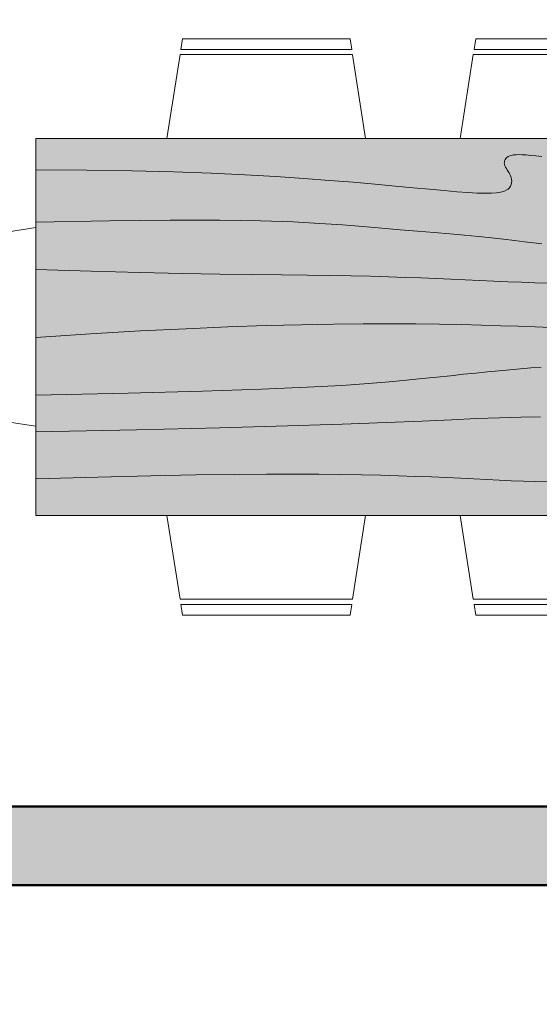
# Model space of a CAD drawing. Units: inches. Extents: x 2419 to 2878, y 1068 to 1713.
# Tile 4 of 20: x 2508 to 2541, y 1286 to 1349. Entities that reach past the tile are written whole.
import ezdxf

# ---------------------------------------------------------------- set-up
doc = ezdxf.new("R2010")
doc.units = ezdxf.units.IN
for name, color, linetype, lineweight in [('A-ANNO-DIMS', 2, 'Continuous', 18), ('A-FLOR-PRKG-PATT', 1, 'Continuous', 13), ('A-FURN', 8, 'Continuous', 18), ('A-FURN-PATT', 254, 'Continuous', 13), ('A-WALL', 7, 'Continuous', 50)]:
    doc.layers.add(name, color=color, linetype=linetype, lineweight=lineweight)
doc.layers.add('A-WALL-PATT', color=18, linetype='Continuous', lineweight=13, true_color=0x000000)
doc.styles.get("Standard").update_dxf_attribs({"font": 'arial.ttf'})
doc.dimstyles.new('ISO-25', dxfattribs={"dimtxt": 12.5, "dimasz": 2.5, "dimexe": 1.25, "dimexo": 0.625, "dimtad": 1, "dimdec": 0, "dimlunit": 4, "dimtxsty": 'Standard', "dimblk": 'ARCHTICK', "dimcen": 2.5, "dimse1": 1, "dimse2": 1, "dimclrd": 4, "dimadec": 0, "dimazin": 0, "dimtfac": 1, "dimtdec": 0, "dimtmove": 0, "dimatfit": 3, "dimfxl": 1, "dimarcsym": 0})

# ---------------------------------------------------------------- blocks, each defined once
blk = doc.blocks.new('Dining Set - 36 x 72 in.')
for p, q in [((-22, 27.5), (-22.1562, 26.50042)), ((-22, 27.5), (-6, 27.5)), ((-5.8437, 26.49966), (-6, 27.5)), ((6, 27.5), (5.8438, 26.50042)), ((6, 27.5), (22, 27.5)), ((-5.8416, 26.5), (-22.1534, 26.5)), ((22.1584, 26.5), (5.8466, 26.5)), ((-22.2343, 26.00059), (-23.4847, 17.99762)), ((-22.2304, 26), (-5.7608, 26)), ((-4.5152, 17.99762), (-5.7655, 25.99926)), ((5.7657, 26.00059), (4.5153, 17.99762)), ((5.7696, 26), (22.2392, 26)), ((36, 18), (-36, 18)), ((-36, 18), (-36, -18)), ((-44.0006, 8.23428), (-35.9976, 9.48474)), ((-35.9976, -9.48476), (-43.9993, -8.2345)), ((-36, -18), (36, -18)), ((-22.2343, -26.0006), (-23.4847, -17.99762)), ((-4.5152, -17.99762), (-5.7655, -25.99928)), ((5.7657, -26.0006), (4.5153, -17.99762)), ((-22.2304, -26), (-5.7608, -26)), ((5.7696, -26), (22.2392, -26)), ((-22, -27.5), (-22.1562, -26.50044)), ((-5.8416, -26.5), (-22.1534, -26.5)), ((-5.8437, -26.49967), (-6, -27.5)), ((6, -27.5), (5.8438, -26.50044)), ((22.1584, -26.5), (5.8466, -26.5)), ((-22, -27.5), (-6, -27.5)), ((6, -27.5), (22, -27.5))]:
    blk.add_line(p, q)
for points in [[(-36, 15), (-31.1772, 14.97754), (-26.8079, 14.91406), (-22.8538, 14.81543), (-19.276, 14.6875), (-16.0362, 14.53613), (-13.0957, 14.36718), (-10.4159, 14.18652), (-7.9583, 14), (-5.6904, 13.81315), (-3.6035, 13.63021), (-1.6954, 13.45508), (0.0365, 13.29166), (1.5945, 13.14388), (2.9811, 13.01562), (4.1988, 12.9108), (5.25, 12.83333), (6.1393, 12.78613), (6.8802, 12.76823), (7.4883, 12.77767), (7.9792, 12.8125), (8.3685, 12.87077), (8.6719, 12.95052), (8.9049, 13.0498), (9.0833, 13.16666), (9.2205, 13.29899), (9.3216, 13.44401), (9.3895, 13.59879), (9.4271, 13.76041), (9.4373, 13.92594), (9.4232, 14.09245), (9.3875, 14.257), (9.3333, 14.41666), (9.2638, 14.56917), (9.1836, 14.71484), (9.0975, 14.85465), (9.0104, 14.98958), (8.9272, 15.1206), (8.8529, 15.2487), (8.7922, 15.37483), (8.75, 15.5), (8.7305, 15.62467), (8.7344, 15.74739), (8.7617, 15.86621), (8.8125, 15.97916), (8.8867, 16.08431), (8.9844, 16.17968), (9.1055, 16.26334), (9.25, 16.33333), (9.4189, 16.38802), (9.6172, 16.42708), (9.8506, 16.45052), (10.125, 16.45833), (10.4463, 16.45052), (10.8203, 16.42708), (11.2529, 16.38802), (11.75, 16.33333), (12.3184, 16.26318)], [(-36, 10), (-28.9766, 10.14274), (-23.1725, 10.20442), (-18.4241, 10.19775), (-14.5677, 10.13541), (-11.4399, 10.03011), (-8.877, 9.89453), (-6.7154, 9.74137), (-4.7917, 9.58333), (-2.9698, 9.43082), (-1.2246, 9.28515), (0.4415, 9.14534), (2.026, 9.01041), (3.5266, 8.87939), (4.9408, 8.7513), (6.266, 8.62516), (7.5, 8.5), (8.6411, 8.37549), (9.6914, 8.2539), (10.6538, 8.13818), (11.5312, 8.03125), (12.3267, 7.93603)], [(-36, 5.5), (-30.7157, 5.3348), (-26.069, 5.20963), (-21.9946, 5.11767), (-18.4271, 5.05208), (-15.3009, 5.00602), (-12.5508, 4.97265), (-10.1112, 4.94515), (-7.9167, 4.91666), (-5.909, 4.88167), (-4.0586, 4.83984), (-2.3429, 4.79215), (-0.7396, 4.73958), (0.7739, 4.6831), (2.22, 4.6237), (3.6213, 4.56233), (5, 4.5), (6.373, 4.43782), (7.7344, 4.3776), (9.0723, 4.32129), (10.375, 4.27083), (11.6309, 4.22819), (12.8281, 4.19531)], [(-36, -1), (-30.7915, -0.6591), (-26.0195, -0.38216), (-21.6519, -0.16284), (-17.6563, 0.00521), (-14.0005, 0.12833), (-10.6523, 0.21289), (-7.5796, 0.26522), (-4.75, 0.29166), (-2.134, 0.29793), (0.2878, 0.28711), (2.5317, 0.26163), (4.6146, 0.22396), (6.5529, 0.17651), (8.3633, 0.12174), (10.0623, 0.06209), (11.6667, 0), (13.1899, -0.06201)], [(-36, -6.5), (-27.1843, -6.31267), (-20.084, -6.1263), (-14.469, -5.9419), (-10.1094, -5.76042), (-6.7752, -5.58285), (-4.2363, -5.41016), (-2.2629, -5.24333), (-0.625, -5.08334), (0.8708, -4.93099), (2.2715, -4.78646), (3.5872, -4.64974), (4.8281, -4.52084), (6.0046, -4.39974), (7.127, -4.28646), (8.2053, -4.18099), (9.25, -4.08334), (10.2705, -3.99382), (11.2734, -3.91407), (12.2647, -3.84603)], [(-36, -10), (-26.4022, -9.81299), (-18.4675, -9.62891), (-11.9839, -9.45069), (-6.7396, -9.28125), (-2.5226, -9.12354), (0.8789, -8.98047), (3.6769, -8.85498), (6.0833, -8.75), (8.2767, -8.66765), (10.3021, -8.60677), (12.1712, -8.56543)], [(-36, -14.5), (-30.0881, -14.33513), (-25.0332, -14.21224), (-20.7312, -14.12647), (-17.0781, -14.07292), (-13.97, -14.04671), (-11.3027, -14.04297), (-8.9724, -14.05681), (-6.875, -14.08334), (-4.9224, -14.11833), (-3.0905, -14.16016), (-1.3709, -14.20785), (0.2448, -14.26042), (1.7647, -14.3169), (3.1973, -14.3763), (4.5507, -14.43767), (5.8333, -14.5), (7.0554, -14.5621), (8.235, -14.62175), (9.3922, -14.67652), (10.5469, -14.72396), (11.7192, -14.76164), (12.929, -14.78711)]]:
    blk.add_lwpolyline(points)
blk = doc.blocks.new('_ArchTick')
at = {"color": 0, "linetype": 'ByBlock', "const_width": 0.15}
blk.add_lwpolyline([(-0.5, -0.5), (0.5, 0.5)], dxfattribs=at)
blk = doc.blocks.new('*D26')
at = {"layer": 'A-ANNO-DIMS', "color": 4, "lineweight": -2, "transparency": 16777216}
for p, q in [((2502.769, 1356.79), (2563.458, 1356.79)), ((2563.458, 1356.79), (2733.724, 1356.79))]:
    blk.add_line(p, q, dxfattribs=at)
at = {"layer": 'Defpoints', "color": 0, "transparency": 16777216}
for p in [(2563.458, 1356.79), (2502.769, 1347.687), (2563.458, 1347.687)]:
    blk.add_point(p, dxfattribs=at)
at = {"layer": 'A-ANNO-DIMS', "color": 4, "lineweight": -2, "transparency": 16777216, "xscale": 2.5, "yscale": 2.5, "zscale": 2.5, "rotation": 180}
blk.add_blockref('_ArchTick', (2502.769, 1356.79), dxfattribs=at)
at = {"layer": 'A-ANNO-DIMS', "color": 4, "lineweight": -2, "transparency": 16777216, "xscale": 2.5, "yscale": 2.5, "zscale": 2.5}
blk.add_blockref('_ArchTick', (2563.458, 1356.79), dxfattribs=at)
at = {"layer": 'A-ANNO-DIMS', "color": 0, "transparency": 16777216, "insert": (2649.841, 1363.878), "char_height": 12.5, "attachment_point": 5}
blk.add_mtext('DINING SET 5\'-0 1/2"', dxfattribs=at)
blk = doc.blocks.new('*D43')
at = {"layer": 'A-ANNO-DIMS', "color": 4, "lineweight": -2, "transparency": 16777216}
blk.add_line((2480.514, 1079.925), (2557.299, 1079.925), dxfattribs=at)
at = {"layer": 'Defpoints', "color": 0, "transparency": 16777216}
for p in [(2480.514, 1408.813), (2557.299, 1408.813), (2557.299, 1079.925)]:
    blk.add_point(p, dxfattribs=at)
at = {"layer": 'A-ANNO-DIMS', "color": 4, "lineweight": -2, "transparency": 16777216, "xscale": 2.5, "yscale": 2.5, "zscale": 2.5, "rotation": 180}
blk.add_blockref('_ArchTick', (2480.514, 1079.925), dxfattribs=at)
at = {"layer": 'A-ANNO-DIMS', "color": 4, "lineweight": -2, "transparency": 16777216, "xscale": 2.5, "yscale": 2.5, "zscale": 2.5}
blk.add_blockref('_ArchTick', (2557.299, 1079.925), dxfattribs=at)
at = {"layer": 'A-ANNO-DIMS', "color": 0, "transparency": 16777216, "insert": (2518.907, 1086.932), "char_height": 12.5, "attachment_point": 5}
blk.add_mtext('6\'-5"', dxfattribs=at)
blk = doc.blocks.new('*D47')
at = {"layer": 'A-ANNO-DIMS', "color": 4, "lineweight": -2, "transparency": 16777216}
for p, q in [((2444.314, 1376.561), (2444.314, 1357.976)), ((2444.314, 1357.976), (2444.314, 1293.048))]:
    blk.add_line(p, q, dxfattribs=at)
at = {"layer": 'Defpoints', "color": 0, "transparency": 16777216}
for p in [(2632.514, 1376.561), (2444.314, 1357.976), (2632.514, 1357.976)]:
    blk.add_point(p, dxfattribs=at)
at = {"layer": 'A-ANNO-DIMS', "color": 4, "lineweight": -2, "transparency": 16777216, "xscale": 2.5, "yscale": 2.5, "zscale": 2.5}
for p, rotation in [((2444.314, 1376.561), 90), ((2444.314, 1357.976), 270)]:
    blk.add_blockref('_ArchTick', p, dxfattribs=dict(at, rotation=rotation))
at = {"layer": 'A-ANNO-DIMS', "color": 0, "transparency": 16777216, "insert": (2437.226, 1324.262), "char_height": 12.5, "attachment_point": 5, "rotation": 90}
blk.add_mtext('1\'-6 1/2"', dxfattribs=at)
blk = doc.blocks.new('*D56')
at = {"layer": 'A-ANNO-DIMS', "color": 4, "lineweight": -2, "transparency": 16777216}
for p, q in [((2480.514, 1079.925), (2503.967, 1079.925)), ((2503.967, 1079.925), (2578.607, 1079.925))]:
    blk.add_line(p, q, dxfattribs=at)
at = {"layer": 'Defpoints', "color": 0, "transparency": 16777216}
for p in [(2480.514, 1507.813), (2503.967, 1494.852), (2503.967, 1079.925)]:
    blk.add_point(p, dxfattribs=at)
at = {"layer": 'A-ANNO-DIMS', "color": 4, "lineweight": -2, "transparency": 16777216, "xscale": 2.5, "yscale": 2.5, "zscale": 2.5, "rotation": 180}
blk.add_blockref('_ArchTick', (2480.514, 1079.925), dxfattribs=at)
at = {"layer": 'A-ANNO-DIMS', "color": 4, "lineweight": -2, "transparency": 16777216, "xscale": 2.5, "yscale": 2.5, "zscale": 2.5}
blk.add_blockref('_ArchTick', (2503.967, 1079.925), dxfattribs=at)
at = {"layer": 'A-ANNO-DIMS', "color": 0, "transparency": 16777216, "insert": (2542.537, 1087.013), "char_height": 12.5, "attachment_point": 5}
blk.add_mtext('1\'-11 1/2"', dxfattribs=at)
blk = doc.blocks.new('*D59')
at = {"layer": 'A-ANNO-DIMS', "color": 4, "lineweight": -2, "transparency": 16777216}
blk.add_line((2480.514, 1079.925), (2589.514, 1079.925), dxfattribs=at)
at = {"layer": 'Defpoints', "color": 0, "transparency": 16777216}
for p in [(2480.514, 1414.813), (2589.514, 1414.813), (2589.514, 1079.925)]:
    blk.add_point(p, dxfattribs=at)
at = {"layer": 'A-ANNO-DIMS', "color": 4, "lineweight": -2, "transparency": 16777216, "xscale": 2.5, "yscale": 2.5, "zscale": 2.5, "rotation": 180}
blk.add_blockref('_ArchTick', (2480.514, 1079.925), dxfattribs=at)
at = {"layer": 'A-ANNO-DIMS', "color": 4, "lineweight": -2, "transparency": 16777216, "xscale": 2.5, "yscale": 2.5, "zscale": 2.5}
blk.add_blockref('_ArchTick', (2589.514, 1079.925), dxfattribs=at)
at = {"layer": 'A-ANNO-DIMS', "color": 0, "transparency": 16777216, "insert": (2535.014, 1086.932), "char_height": 12.5, "attachment_point": 5}
blk.add_mtext('9\'-1"', dxfattribs=at)

msp = doc.modelspace()

# ---------------------------------------------------------------- hatches: boundary and pattern name
at = {"layer": 'A-FLOR-PRKG-PATT'}
h = msp.add_hatch(color=256, dxfattribs=at)
h.dxf.hatch_style = 1
edge = h.paths.add_edge_path()
edge.add_ellipse((2561.374, 1279.453), major_axis=(3.988, 0), ratio=0.842304, start_angle=0.64655, end_angle=90)
edge.add_line((2561.374, 1282.813), (2511.571, 1282.813))
edge.add_ellipse((2511.571, 1279.453), major_axis=(3.988, 0), ratio=0.842304, start_angle=90, end_angle=179.35345)
edge.add_ellipse((10560.892, 1188.617), major_axis=(-8054.031, 0), ratio=0.84230387, start_angle=-0.6465541, end_angle=-0.6282372)
edge.add_ellipse((2509.23, 1276.906), major_axis=(1.687, 0), ratio=0.842304, start_angle=179.37176, end_angle=248.46476)
edge.add_ellipse((10560.329, 1188.617), major_axis=(8052.293, 0), ratio=0.84230387, start_angle=179.3534459, end_angle=179.3813568, ccw=False)
edge.add_ellipse((2511.008, 1279.453), major_axis=(2.25, 0), ratio=0.842304, start_angle=90, end_angle=179.35345, ccw=False)
edge.add_line((2511.008, 1281.348), (2561.936, 1281.348))
edge.add_ellipse((2561.936, 1279.453), major_axis=(-2.25, 0), ratio=0.842304, start_angle=180.64655, end_angle=270, ccw=False)
edge.add_ellipse((-5487.385, 1188.617), major_axis=(8052.293, 0), ratio=0.84230387, start_angle=0.5282715, end_angle=0.6465541, ccw=False)
edge.add_ellipse((2563.715, 1276.906), major_axis=(-1.687, 0), ratio=0.842304, start_angle=111.53524, end_angle=180.62824)
edge.add_ellipse((-5487.947, 1188.617), major_axis=(-8054.031, 0), ratio=0.84230387, start_angle=180.6282372, end_angle=180.6465541)
edge = h.paths.add_edge_path()
edge.add_ellipse((2564.908, 1261.91), major_axis=(-1.125, 0), ratio=0.842304, start_angle=180, end_angle=270)
edge.add_line((2564.908, 1262.857), (2564.426, 1262.857))
edge.add_ellipse((-5487.385, 1188.617), major_axis=(8052.293, 0), ratio=0.84230387, start_angle=0.3838668, end_angle=0.5282715, ccw=False)
edge.add_line((2564.654, 1242.564), (2564.908, 1242.564))
edge.add_ellipse((2564.908, 1243.512), major_axis=(-1.125, 0), ratio=0.842304, start_angle=90, end_angle=180)
edge.add_line((2566.033, 1243.512), (2566.033, 1261.91))
edge = h.paths.add_edge_path()
edge.add_ellipse((2564.908, 1174.989), major_axis=(1.125, 0), ratio=0.842304, start_angle=0, end_angle=90)
edge.add_line((2564.908, 1175.936), (2564.894, 1175.936))
edge.add_ellipse((-5487.385, 1188.617), major_axis=(8052.293, 0), ratio=0.84230387, start_angle=-0.1349866, end_angle=-0.0902291, ccw=False)
edge.add_ellipse((2163.343, 1170.913), major_axis=(401.537, 0), ratio=0.8423039, start_angle=-2.17995, end_angle=-0.13561, ccw=False)
edge.add_line((2564.47, 1155.643), (2564.908, 1155.643))
edge.add_ellipse((2564.908, 1156.591), major_axis=(-1.125, 0), ratio=0.842304, start_angle=90, end_angle=180)
edge.add_line((2566.033, 1156.591), (2566.033, 1174.989))
h.paths.add_polyline_path([(2574.476, 1207.448), (2633.94, 1207.448), (2633.94, 1217.366), (2574.476, 1217.366)], flags=9)
h.paths.add_polyline_path([(2574.454, 1217.828), (2610.472, 1217.828), (2610.472, 1227.879), (2574.454, 1227.879)], flags=9)
h.paths.add_polyline_path([(2672.426, 1304.02), (2718.617, 1304.02), (2718.617, 1313.939), (2672.426, 1313.939)], flags=9)
h.paths.add_polyline_path([(2672.404, 1314.4), (2750.128, 1314.4), (2750.128, 1324.451), (2672.404, 1324.451)], flags=9)
h.paths.add_polyline_path([(2500.432, 1374.444), (2544.803, 1374.444), (2544.803, 1384.362), (2500.432, 1384.362)], flags=9)
h.paths.add_polyline_path([(2500.41, 1384.824), (2566.075, 1384.824), (2566.075, 1394.875), (2500.41, 1394.875)], flags=9)
h.paths.add_polyline_path([(2738.933, 1376.749), (2778.273, 1376.749), (2778.273, 1386.667), (2738.933, 1386.667)], flags=9)
h.paths.add_polyline_path([(2659.12, 1357.8), (2703.492, 1357.8), (2703.492, 1367.718), (2659.12, 1367.718)], flags=9)
h.paths.add_polyline_path([(2659.098, 1368.18), (2694.114, 1368.18), (2694.114, 1378.23), (2659.098, 1378.23)], flags=9)
h.paths.add_polyline_path([(2730.123, 1466.067), (2769.463, 1466.067), (2769.463, 1475.986), (2730.123, 1475.986)], flags=9)
h.paths.add_polyline_path([(2730.101, 1476.447), (2765.117, 1476.447), (2765.117, 1486.498), (2730.101, 1486.498)], flags=9)
h.paths.add_polyline_path([(2730.382, 1518.647), (2761.48, 1518.647), (2761.48, 1528.566), (2730.382, 1528.566)], flags=9)
h.paths.add_polyline_path([(2730.361, 1529.028), (2780.958, 1529.028), (2780.958, 1539.072), (2730.361, 1539.072)], flags=9)
h.paths.add_polyline_path([(2629.32, 1455.189), (2688.784, 1455.189), (2688.784, 1465.107), (2629.32, 1465.107)], flags=9)
h.paths.add_polyline_path([(2629.298, 1465.569), (2681.902, 1465.569), (2681.902, 1475.62), (2629.298, 1475.62)], flags=9)
h.paths.add_polyline_path([(2513.229, 1456.484), (2562.631, 1456.484), (2562.631, 1466.402), (2513.229, 1466.402)], flags=9)
h.paths.add_polyline_path([(2513.208, 1466.865), (2556.26, 1466.865), (2556.26, 1476.909), (2513.208, 1476.909)], flags=9)
h.paths.add_polyline_path([(2488.87, 1521.538), (2519.968, 1521.538), (2519.968, 1531.456), (2488.87, 1531.456)], flags=9)
h.paths.add_polyline_path([(2536.549, 1543.507), (2580.923, 1543.507), (2580.923, 1553.432), (2536.549, 1553.432)], flags=9)
h.paths.add_polyline_path([(2536.557, 1553.921), (2573.525, 1553.921), (2573.525, 1563.8), (2536.557, 1563.8)], flags=9)
at = {"layer": 'A-FURN-PATT'}
h = msp.add_hatch(color=256, dxfattribs=at)
h.dxf.hatch_style = 1
h.paths.add_polyline_path([(2541.329, 1340.193), (2541.763, 1340.136), (2542.26, 1340.071), (2542.829, 1339.996), (2543.477, 1339.914), (2544.213, 1339.825), (2545.044, 1339.73), (2545.979, 1339.628), (2547.025, 1339.521), (2548.178, 1339.41), (2549.434, 1339.295), (2550.79, 1339.177), (2552.241, 1339.056), (2553.783, 1338.933), (2555.412, 1338.808), (2557.123, 1338.683), (2557.123, 1341.351), (2509.104, 1341.351), (2509.104, 1339.35), (2512.321, 1339.335), (2515.235, 1339.293), (2517.872, 1339.227), (2520.258, 1339.142), (2522.419, 1339.041), (2524.38, 1338.928), (2526.167, 1338.808), (2527.806, 1338.683), (2529.318, 1338.559), (2530.71, 1338.437), (2531.983, 1338.32), (2533.138, 1338.211), (2534.177, 1338.112), (2535.102, 1338.027), (2535.914, 1337.957), (2536.615, 1337.905), (2537.208, 1337.874), (2537.702, 1337.862), (2538.108, 1337.868), (2538.435, 1337.891), (2538.695, 1337.93), (2538.897, 1337.983), (2539.052, 1338.05), (2539.171, 1338.128), (2539.263, 1338.216), (2539.33, 1338.313), (2539.376, 1338.416), (2539.401, 1338.524), (2539.407, 1338.634), (2539.398, 1338.745), (2539.374, 1338.855), (2539.338, 1338.961), (2539.292, 1339.063), (2539.238, 1339.16), (2539.211, 1339.204), (2538.872, 1339.739), (2539.045, 1340.125), (2539.381, 1340.287), (2539.76, 1340.325), (2540.185, 1340.315), (2540.752, 1340.264)])
h.paths.add_polyline_path([(2557.123, 1329.334), (2556.881, 1329.353), (2556.861, 1329.358), (2556.848, 1329.36), (2556.516, 1329.438), (2556.428, 1329.458), (2556.199, 1329.504), (2555.916, 1329.558), (2555.589, 1329.615), (2555.23, 1329.673), (2554.848, 1329.728), (2554.455, 1329.778), (2554.061, 1329.819), (2553.677, 1329.847), (2553.311, 1329.86), (2552.963, 1329.859), (2552.628, 1329.845), (2552.301, 1329.819), (2551.98, 1329.783), (2551.66, 1329.737), (2551.338, 1329.684), (2551.009, 1329.624), (2550.353, 1329.499), (2549.707, 1329.384), (2549.089, 1329.301), (2548.61, 1329.249), (2548.085, 1329.208), (2547.508, 1329.18), (2546.875, 1329.166), (2546.185, 1329.167), (2545.44, 1329.179), (2544.639, 1329.201), (2543.783, 1329.23), (2542.873, 1329.266), (2541.91, 1329.305), (2540.894, 1329.346), (2539.824, 1329.388), (2538.691, 1329.428), (2537.484, 1329.464), (2536.191, 1329.496), (2534.802, 1329.521), (2533.305, 1329.538), (2531.69, 1329.545), (2529.946, 1329.541), (2528.058, 1329.523), (2526.009, 1329.488), (2523.776, 1329.432), (2521.338, 1329.35), (2518.673, 1329.238), (2515.761, 1329.092), (2512.578, 1328.907), (2509.104, 1328.68), (2509.104, 1325.012), (2514.984, 1325.136), (2519.719, 1325.261), (2523.464, 1325.384), (2526.371, 1325.505), (2528.595, 1325.623), (2530.288, 1325.738), (2531.604, 1325.85), (2532.697, 1325.956), (2533.694, 1326.058), (2534.628, 1326.154), (2535.506, 1326.245), (2536.333, 1326.331), (2537.118, 1326.412), (2537.867, 1326.488), (2538.586, 1326.558), (2539.282, 1326.623), (2539.963, 1326.683), (2540.632, 1326.736), (2541.293, 1326.782), (2541.95, 1326.818), (2542.607, 1326.844), (2543.268, 1326.858), (2543.937, 1326.859), (2544.618, 1326.846), (2545.312, 1326.817), (2546.015, 1326.775), (2546.719, 1326.721), (2547.418, 1326.658), (2548.103, 1326.587), (2548.768, 1326.509), (2549.406, 1326.428), (2550.009, 1326.345), (2550.572, 1326.262), (2551.1, 1326.179), (2551.597, 1326.097), (2552.069, 1326.015), (2552.521, 1325.935), (2552.959, 1325.857), (2553.389, 1325.78), (2553.816, 1325.706), (2554.244, 1325.636), (2554.672, 1325.573), (2555.099, 1325.524), (2555.521, 1325.494), (2555.937, 1325.489), (2556.344, 1325.515), (2556.74, 1325.576), (2557.123, 1325.678)])
h.paths.add_polyline_path([(2557.123, 1335.349), (2555.251, 1335.701), (2553.623, 1336.012), (2552.215, 1336.285), (2551.006, 1336.526), (2549.972, 1336.74), (2549.092, 1336.931), (2548.343, 1337.105), (2547.702, 1337.266), (2547.15, 1337.418), (2546.674, 1337.56), (2546.265, 1337.69), (2545.913, 1337.805), (2545.61, 1337.903), (2545.346, 1337.981), (2545.111, 1338.039), (2544.896, 1338.072), (2544.693, 1338.08), (2544.502, 1338.065), (2544.326, 1338.029), (2544.166, 1337.975), (2544.025, 1337.905), (2543.903, 1337.822), (2543.804, 1337.729), (2543.729, 1337.627), (2543.679, 1337.521), (2543.653, 1337.409), (2543.649, 1337.294), (2543.666, 1337.176), (2543.701, 1337.055), (2543.752, 1336.932), (2543.818, 1336.808), (2543.895, 1336.683), (2543.983, 1336.558), (2544.078, 1336.433), (2544.175, 1336.307), (2544.271, 1336.182), (2544.361, 1336.057), (2544.442, 1335.932), (2544.511, 1335.807), (2544.562, 1335.682), (2544.594, 1335.557), (2544.605, 1335.434), (2544.597, 1335.313), (2544.569, 1335.196), (2544.524, 1335.084), (2544.461, 1334.979), (2544.381, 1334.881), (2544.284, 1334.793), (2544.172, 1334.715), (2544.039, 1334.648), (2543.884, 1334.593), (2543.701, 1334.55), (2543.487, 1334.52), (2543.237, 1334.504), (2542.949, 1334.502), (2542.617, 1334.515), (2542.239, 1334.543), (2541.812, 1334.585), (2541.334, 1334.639), (2540.804, 1334.703), (2540.219, 1334.774), (2539.577, 1334.851), (2538.876, 1334.932), (2538.115, 1335.015), (2537.292, 1335.099), (2536.409, 1335.183), (2535.465, 1335.268), (2534.465, 1335.356), (2533.408, 1335.446), (2532.297, 1335.539), (2531.133, 1335.636), (2529.918, 1335.738), (2528.635, 1335.843), (2527.193, 1335.945), (2525.484, 1336.036), (2523.398, 1336.106), (2520.826, 1336.148), (2517.659, 1336.152), (2513.788, 1336.111), (2509.104, 1336.016), (2509.104, 1333.015), (2512.629, 1332.904), (2515.728, 1332.821), (2518.445, 1332.76), (2520.824, 1332.716), (2522.909, 1332.685), (2524.743, 1332.663), (2526.37, 1332.645), (2527.834, 1332.626), (2529.173, 1332.602), (2530.407, 1332.574), (2531.551, 1332.542), (2532.62, 1332.507), (2533.63, 1332.47), (2534.594, 1332.43), (2535.529, 1332.389), (2536.448, 1332.348), (2537.364, 1332.306), (2538.272, 1332.266), (2539.164, 1332.228), (2540.033, 1332.195), (2540.87, 1332.166), (2541.669, 1332.144), (2542.42, 1332.13), (2543.117, 1332.125), (2543.754, 1332.131), (2544.33, 1332.146), (2544.851, 1332.172), (2545.32, 1332.209), (2545.738, 1332.256), (2546.111, 1332.313), (2546.44, 1332.381), (2546.73, 1332.459), (2546.983, 1332.547), (2547.206, 1332.644), (2547.402, 1332.747), (2547.577, 1332.855), (2547.737, 1332.965), (2547.886, 1333.076), (2548.031, 1333.186), (2548.175, 1333.292), (2548.324, 1333.394), (2548.48, 1333.489), (2548.645, 1333.576), (2548.821, 1333.654), (2549.01, 1333.721), (2549.214, 1333.777), (2549.435, 1333.82), (2549.675, 1333.848), (2549.936, 1333.861), (2550.215, 1333.859), (2550.511, 1333.843), (2550.822, 1333.813), (2551.146, 1333.771), (2551.481, 1333.715), (2551.825, 1333.648), (2552.176, 1333.57), (2552.537, 1333.481), (2552.926, 1333.379), (2553.365, 1333.262), (2553.878, 1333.126), (2554.488, 1332.969), (2555.217, 1332.789), (2556.087, 1332.583), (2557.123, 1332.348)])
h.paths.add_polyline_path([(2543.679, 1337.521), (2543.729, 1337.627), (2543.804, 1337.729), (2543.903, 1337.822), (2544.025, 1337.905), (2544.166, 1337.975), (2544.326, 1338.029), (2544.502, 1338.065), (2544.693, 1338.08), (2544.896, 1338.072), (2545.111, 1338.039), (2545.346, 1337.981), (2545.61, 1337.903), (2545.913, 1337.805), (2546.265, 1337.69), (2546.674, 1337.56), (2547.15, 1337.418), (2547.702, 1337.266), (2548.343, 1337.105), (2549.092, 1336.931), (2549.972, 1336.74), (2551.006, 1336.526), (2552.215, 1336.285), (2553.623, 1336.012), (2555.251, 1335.701), (2557.123, 1335.349), (2557.123, 1338.683), (2555.412, 1338.808), (2553.783, 1338.933), (2552.241, 1339.056), (2550.79, 1339.177), (2549.434, 1339.295), (2548.178, 1339.41), (2547.025, 1339.521), (2545.979, 1339.628), (2545.044, 1339.73), (2544.213, 1339.825), (2543.477, 1339.914), (2542.829, 1339.996), (2542.26, 1340.071), (2541.763, 1340.136), (2541.329, 1340.193), (2540.95, 1340.24), (2540.618, 1340.276), (2540.33, 1340.302), (2540.08, 1340.318), (2539.866, 1340.323), (2539.683, 1340.318), (2539.527, 1340.302), (2539.395, 1340.276), (2539.282, 1340.24), (2539.186, 1340.193), (2539.105, 1340.137), (2539.04, 1340.073), (2538.991, 1340.003), (2538.957, 1339.928), (2538.939, 1339.849), (2538.936, 1339.767), (2538.949, 1339.684), (2538.977, 1339.6), (2539.018, 1339.516), (2539.067, 1339.431), (2539.123, 1339.343), (2539.222, 1339.189), (2539.323, 1339.007), (2539.374, 1338.855), (2539.398, 1338.745), (2539.407, 1338.634), (2539.401, 1338.524), (2539.376, 1338.416), (2539.33, 1338.313), (2539.263, 1338.216), (2539.171, 1338.128), (2539.052, 1338.05), (2538.897, 1337.983), (2538.695, 1337.93), (2538.435, 1337.891), (2538.108, 1337.868), (2537.702, 1337.862), (2537.208, 1337.874), (2536.615, 1337.905), (2535.914, 1337.957), (2535.102, 1338.027), (2534.177, 1338.112), (2533.138, 1338.211), (2531.983, 1338.32), (2530.71, 1338.437), (2529.318, 1338.559), (2527.806, 1338.683), (2526.167, 1338.808), (2524.38, 1338.928), (2522.419, 1339.041), (2520.258, 1339.142), (2517.872, 1339.227), (2515.235, 1339.293), (2512.321, 1339.335), (2509.104, 1339.35), (2509.104, 1336.016), (2513.788, 1336.111), (2517.659, 1336.152), (2520.826, 1336.148), (2523.398, 1336.106), (2525.484, 1336.036), (2527.193, 1335.945), (2528.635, 1335.843), (2529.918, 1335.738), (2531.133, 1335.636), (2532.297, 1335.539), (2533.408, 1335.446), (2534.465, 1335.356), (2535.465, 1335.268), (2536.409, 1335.183), (2537.292, 1335.099), (2538.115, 1335.015), (2538.876, 1334.932), (2539.577, 1334.851), (2540.219, 1334.774), (2540.804, 1334.703), (2541.334, 1334.639), (2541.812, 1334.585), (2542.239, 1334.543), (2542.617, 1334.515), (2542.949, 1334.502), (2543.237, 1334.504), (2543.487, 1334.52), (2543.701, 1334.55), (2543.884, 1334.593), (2544.039, 1334.648), (2544.172, 1334.715), (2544.284, 1334.793), (2544.381, 1334.881), (2544.461, 1334.979), (2544.524, 1335.084), (2544.569, 1335.196), (2544.597, 1335.313), (2544.605, 1335.434), (2544.594, 1335.557), (2544.562, 1335.682), (2544.511, 1335.807), (2544.442, 1335.932), (2544.361, 1336.057), (2544.271, 1336.182), (2544.175, 1336.307), (2544.078, 1336.433), (2543.983, 1336.558), (2543.895, 1336.683), (2543.818, 1336.808), (2543.752, 1336.932), (2543.701, 1337.055), (2543.666, 1337.176), (2543.649, 1337.294), (2543.653, 1337.409)])
h.paths.add_polyline_path([(2557.123, 1332.348), (2556.087, 1332.583), (2555.217, 1332.789), (2554.488, 1332.969), (2553.878, 1333.126), (2553.365, 1333.262), (2552.926, 1333.379), (2552.537, 1333.481), (2552.176, 1333.57), (2551.825, 1333.648), (2551.481, 1333.715), (2551.146, 1333.771), (2550.822, 1333.813), (2550.511, 1333.843), (2550.215, 1333.859), (2549.936, 1333.861), (2549.675, 1333.848), (2549.435, 1333.82), (2549.214, 1333.777), (2549.01, 1333.721), (2548.821, 1333.654), (2548.645, 1333.576), (2548.48, 1333.489), (2548.324, 1333.394), (2548.175, 1333.292), (2548.031, 1333.186), (2547.886, 1333.076), (2547.737, 1332.965), (2547.577, 1332.855), (2547.402, 1332.747), (2547.206, 1332.644), (2546.983, 1332.547), (2546.73, 1332.459), (2546.44, 1332.381), (2546.111, 1332.313), (2545.738, 1332.256), (2545.32, 1332.209), (2544.851, 1332.172), (2544.33, 1332.146), (2543.754, 1332.131), (2543.117, 1332.125), (2542.42, 1332.13), (2541.669, 1332.144), (2540.87, 1332.166), (2540.033, 1332.195), (2539.164, 1332.228), (2538.272, 1332.266), (2537.364, 1332.306), (2536.448, 1332.348), (2535.529, 1332.389), (2534.594, 1332.43), (2533.63, 1332.47), (2532.62, 1332.507), (2531.551, 1332.542), (2530.407, 1332.574), (2529.173, 1332.602), (2527.834, 1332.626), (2526.37, 1332.645), (2524.743, 1332.663), (2522.909, 1332.685), (2520.824, 1332.716), (2518.445, 1332.76), (2515.728, 1332.821), (2512.629, 1332.904), (2509.104, 1333.015), (2509.104, 1328.68), (2512.578, 1328.907), (2515.761, 1329.092), (2518.673, 1329.238), (2521.338, 1329.35), (2523.776, 1329.432), (2526.009, 1329.488), (2528.058, 1329.523), (2529.946, 1329.541), (2531.69, 1329.545), (2533.305, 1329.538), (2534.802, 1329.521), (2536.191, 1329.496), (2537.484, 1329.464), (2538.691, 1329.428), (2539.824, 1329.388), (2540.894, 1329.346), (2541.91, 1329.305), (2542.873, 1329.266), (2543.783, 1329.23), (2544.639, 1329.201), (2545.44, 1329.179), (2546.185, 1329.167), (2546.875, 1329.166), (2547.508, 1329.18), (2548.085, 1329.208), (2548.61, 1329.249), (2549.089, 1329.301), (2549.529, 1329.36), (2549.936, 1329.425), (2550.314, 1329.492), (2550.67, 1329.56), (2551.009, 1329.624), (2551.338, 1329.684), (2551.66, 1329.737), (2551.98, 1329.783), (2552.301, 1329.819), (2552.628, 1329.845), (2552.963, 1329.859), (2553.311, 1329.86), (2553.677, 1329.847), (2554.061, 1329.819), (2554.455, 1329.778), (2554.848, 1329.728), (2555.23, 1329.673), (2555.589, 1329.615), (2555.916, 1329.558), (2556.199, 1329.504), (2556.428, 1329.458), (2556.596, 1329.421), (2556.712, 1329.393), (2556.792, 1329.374), (2556.848, 1329.36), (2556.895, 1329.352), (2556.948, 1329.348), (2557.019, 1329.347), (2557.123, 1329.346)])
h.paths.add_polyline_path([(2557.123, 1323.011), (2556.483, 1323.018), (2555.818, 1323.039), (2555.136, 1323.071), (2554.441, 1323.111), (2553.741, 1323.159), (2553.043, 1323.21), (2552.352, 1323.263), (2551.676, 1323.316), (2551.018, 1323.367), (2550.371, 1323.415), (2549.725, 1323.46), (2549.071, 1323.501), (2548.398, 1323.538), (2547.698, 1323.57), (2546.96, 1323.599), (2546.174, 1323.622), (2545.331, 1323.64), (2544.423, 1323.652), (2543.442, 1323.655), (2542.381, 1323.65), (2541.231, 1323.634), (2539.984, 1323.606), (2538.633, 1323.566), (2537.171, 1323.511), (2535.566, 1323.441), (2533.7, 1323.357), (2531.431, 1323.262), (2528.619, 1323.157), (2525.121, 1323.044), (2520.797, 1322.925), (2515.505, 1322.802), (2509.104, 1322.677), (2509.104, 1319.676), (2513.047, 1319.786), (2516.418, 1319.868), (2519.287, 1319.925), (2521.724, 1319.961), (2523.797, 1319.978), (2525.575, 1319.981), (2527.13, 1319.972), (2528.528, 1319.954), (2529.831, 1319.931), (2531.052, 1319.903), (2532.199, 1319.871), (2533.277, 1319.836), (2534.29, 1319.798), (2535.246, 1319.759), (2536.148, 1319.718), (2537.004, 1319.676), (2537.819, 1319.635), (2538.606, 1319.595), (2539.377, 1319.558), (2540.147, 1319.527), (2540.929, 1319.502), (2541.736, 1319.485), (2542.581, 1319.477), (2543.479, 1319.482), (2544.447, 1319.5), (2545.528, 1319.539), (2546.772, 1319.608), (2548.227, 1319.714), (2549.941, 1319.866), (2551.962, 1320.072), (2554.34, 1320.339), (2557.123, 1320.677)], flags=17)
h.paths.add_polyline_path([(2557.123, 1325.678), (2556.74, 1325.576), (2556.344, 1325.515), (2555.937, 1325.489), (2555.521, 1325.494), (2555.099, 1325.524), (2554.672, 1325.573), (2554.244, 1325.636), (2553.816, 1325.706), (2553.389, 1325.78), (2552.959, 1325.857), (2552.521, 1325.935), (2552.069, 1326.015), (2551.597, 1326.097), (2551.1, 1326.179), (2550.572, 1326.262), (2550.009, 1326.345), (2549.406, 1326.428), (2548.768, 1326.509), (2548.103, 1326.587), (2547.418, 1326.658), (2546.719, 1326.721), (2546.015, 1326.775), (2545.312, 1326.817), (2544.618, 1326.846), (2543.937, 1326.859), (2543.268, 1326.858), (2542.607, 1326.844), (2541.95, 1326.818), (2541.293, 1326.782), (2540.632, 1326.736), (2539.963, 1326.683), (2539.282, 1326.623), (2538.586, 1326.558), (2537.867, 1326.488), (2537.118, 1326.412), (2536.333, 1326.331), (2535.506, 1326.245), (2534.628, 1326.154), (2533.694, 1326.058), (2532.697, 1325.956), (2531.604, 1325.85), (2530.288, 1325.738), (2528.595, 1325.623), (2526.371, 1325.505), (2523.464, 1325.384), (2519.719, 1325.261), (2514.984, 1325.136), (2509.104, 1325.012), (2509.104, 1319.676), (2513.047, 1319.786), (2516.418, 1319.868), (2519.287, 1319.925), (2521.724, 1319.961), (2523.797, 1319.978), (2525.575, 1319.981), (2527.13, 1319.972), (2528.528, 1319.954), (2529.831, 1319.931), (2531.052, 1319.903), (2532.199, 1319.871), (2533.277, 1319.836), (2534.29, 1319.798), (2535.246, 1319.759), (2536.148, 1319.718), (2537.004, 1319.676), (2537.819, 1319.635), (2538.606, 1319.595), (2539.377, 1319.558), (2540.147, 1319.527), (2540.929, 1319.502), (2541.736, 1319.485), (2542.581, 1319.477), (2543.479, 1319.482), (2544.447, 1319.5), (2545.528, 1319.539), (2546.772, 1319.608), (2548.227, 1319.714), (2549.941, 1319.866), (2551.962, 1320.072), (2554.34, 1320.339), (2557.123, 1320.677)])
h.paths.add_polyline_path([(2557.123, 1320.677), (2554.34, 1320.339), (2551.962, 1320.072), (2549.941, 1319.866), (2548.227, 1319.714), (2546.772, 1319.608), (2545.528, 1319.539), (2544.447, 1319.5), (2543.479, 1319.482), (2542.581, 1319.477), (2541.736, 1319.485), (2540.929, 1319.502), (2540.147, 1319.527), (2539.377, 1319.558), (2538.606, 1319.595), (2537.819, 1319.635), (2537.004, 1319.676), (2536.148, 1319.718), (2535.246, 1319.759), (2534.29, 1319.798), (2533.277, 1319.836), (2532.199, 1319.871), (2531.052, 1319.903), (2529.831, 1319.931), (2528.528, 1319.954), (2527.13, 1319.972), (2525.575, 1319.981), (2523.797, 1319.978), (2521.724, 1319.961), (2519.287, 1319.925), (2516.418, 1319.868), (2513.047, 1319.786), (2509.104, 1319.676), (2509.104, 1317.342), (2557.123, 1317.342)])
h = msp.add_hatch(color=256, dxfattribs=at)
h.dxf.hatch_style = 1
h.paths.add_polyline_path([(2557.123, 1323.011), (2556.483, 1323.018), (2555.818, 1323.039), (2555.136, 1323.071), (2554.441, 1323.111), (2553.741, 1323.159), (2553.043, 1323.21), (2552.352, 1323.263), (2551.676, 1323.316), (2551.018, 1323.367), (2550.371, 1323.415), (2549.725, 1323.46), (2549.071, 1323.501), (2548.398, 1323.538), (2547.698, 1323.57), (2546.96, 1323.599), (2546.174, 1323.622), (2545.331, 1323.64), (2544.423, 1323.652), (2543.442, 1323.655), (2542.381, 1323.65), (2541.231, 1323.634), (2539.984, 1323.606), (2538.633, 1323.566), (2537.171, 1323.511), (2535.566, 1323.441), (2533.7, 1323.357), (2531.431, 1323.262), (2528.619, 1323.157), (2525.121, 1323.044), (2520.797, 1322.925), (2515.505, 1322.802), (2509.104, 1322.677), (2509.104, 1319.676), (2513.047, 1319.786), (2516.418, 1319.868), (2519.287, 1319.925), (2521.724, 1319.961), (2523.797, 1319.978), (2525.575, 1319.981), (2527.13, 1319.972), (2528.528, 1319.954), (2529.831, 1319.931), (2531.052, 1319.903), (2532.199, 1319.871), (2533.277, 1319.836), (2534.29, 1319.798), (2535.246, 1319.759), (2536.148, 1319.718), (2537.004, 1319.676), (2537.819, 1319.635), (2538.606, 1319.595), (2539.377, 1319.558), (2540.147, 1319.527), (2540.929, 1319.502), (2541.736, 1319.485), (2542.581, 1319.477), (2543.479, 1319.482), (2544.447, 1319.5), (2545.528, 1319.539), (2546.772, 1319.608), (2548.227, 1319.714), (2549.941, 1319.866), (2551.962, 1320.072), (2554.34, 1320.339), (2557.123, 1320.677)])
at = {"layer": 'A-WALL-PATT'}
h = msp.add_hatch(color=256, dxfattribs=at)
h.dxf.hatch_style = 1
h.paths.add_polyline_path([(2780.514, 1577.813), (2471.514, 1577.813), (2471.514, 1121.813), (2780.514, 1121.813)])
h.paths.add_polyline_path([(2480.514, 1568.813), (2771.514, 1568.813), (2771.514, 1130.813), (2480.514, 1130.813)], flags=16)
h.paths.add_polyline_path([(2528.514, 1568.813), (2528.514, 1512.813), (2594.514, 1512.813), (2594.514, 1414.813), (2596.568, 1414.813), (2596.568, 1441.609), (2597.816, 1441.609), (2597.816, 1441.582, -0.384016), (2625.035, 1414.813), (2725.514, 1414.813), (2725.514, 1567.545), (2728.302, 1567.545), (2746.887, 1567.545), (2746.887, 1566.732), (2746.87, 1566.732, -0.367216), (2730.514, 1549.092), (2730.514, 1512.813), (2750.853, 1512.813), (2750.853, 1510.025, -0.401453), (2733.081, 1491.458), (2733.081, 1491.44), (2732.268, 1491.44), (2732.268, 1507.813), (2730.514, 1507.813), (2730.514, 1408.813), (2736.514, 1408.813), (2736.514, 1349.813), (2632.514, 1349.813), (2632.514, 1408.813), (2528.514, 1408.813), (2528.514, 1414.813), (2503.967, 1414.813), (2503.967, 1494.852), (2558.379, 1494.852), (2558.379, 1507.813), (2529.965, 1507.813, -0.414214), (2530.821, 1506.957), (2530.821, 1497.257, -0.414214), (2529.965, 1496.401), (2514.559, 1496.401, -0.414214), (2513.703, 1497.257), (2513.703, 1506.957, -0.414214), (2514.559, 1507.813), (2528.514, 1507.813), (2528.514, 1512.813), (2480.514, 1512.813)], flags=0)
h.paths.add_polyline_path([(2516.262, 1507.813), (2528.262, 1507.813), (2528.262, 1505.813), (2523.417, 1505.813), (2524.074, 1504.675), (2529.394, 1504.675, -0.414214), (2529.965, 1504.104), (2529.965, 1497.828, -0.414214), (2529.394, 1497.257), (2515.13, 1497.257, -0.414214), (2514.559, 1497.828), (2514.559, 1504.104, -0.414214), (2515.13, 1504.675), (2520.689, 1504.675), (2521.342, 1505.813), (2516.262, 1505.813)], flags=0)
h.paths.add_polyline_path([(2522.016, 1505.531), (2522.817, 1507.318, -0.65506), (2522.254, 1506.063), (2522.195, 1505.93), (2522.425, 1505.531)], flags=0)
h.paths.add_polyline_path([(2522.833, 1500.966, -1), (2521.691, 1500.966, -1)], flags=0)
h.paths.add_polyline_path([(2522.547, 1500.966, -1), (2521.977, 1500.966, -1)], flags=0)
h.paths.add_polyline_path([(2482.005, 1470.633), (2499.894, 1470.633), (2499.894, 1448.272), (2482.005, 1448.272), (2482.005, 1452.744), (2481.26, 1452.744), (2481.26, 1449.763), (2480.514, 1449.763), (2480.514, 1469.142), (2481.26, 1469.142), (2481.26, 1466.16), (2482.005, 1466.16)], flags=0)
h.paths.add_polyline_path([(2488.713, 1466.16, -1), (2484.241, 1466.16, -1)], flags=0)
h.paths.add_polyline_path([(2496.167, 1466.16, -1), (2490.204, 1466.16, -1)], flags=0)
h.paths.add_polyline_path([(2487.968, 1466.16, -1), (2484.987, 1466.16, -1)], flags=0)
h.paths.add_polyline_path([(2495.422, 1466.16, -1), (2490.949, 1466.16, -1)], flags=0)
h.paths.add_polyline_path([(2487.223, 1466.16, -1), (2485.732, 1466.16, -1)], flags=0)
h.paths.add_polyline_path([(2494.676, 1466.16, -1), (2491.695, 1466.16, -1)], flags=0)
h.paths.add_polyline_path([(2499.108, 1468.005, -1), (2497.977, 1468.005, -1)], flags=0)
h.paths.add_polyline_path([(2493.931, 1466.16, -1), (2492.44, 1466.16, -1)], flags=0)
h.paths.add_polyline_path([(2499.372, 1463.71, -1), (2498.166, 1463.71, -1)], flags=0)
h.paths.add_polyline_path([(2484.241, 1461.688), (2496.167, 1461.688), (2496.167, 1457.216), (2484.241, 1457.216)], flags=0)
h.paths.add_polyline_path([(2484.987, 1460.943), (2495.422, 1460.943), (2495.422, 1457.961), (2484.987, 1457.961)], flags=0)
h.paths.add_polyline_path([(2586.88, 1510.025), (2587.693, 1510.025), (2587.693, 1491.44), (2586.88, 1491.44)], flags=0)
h.paths.add_polyline_path([(2499.259, 1459.415, -1), (2498.203, 1459.415, -1)], flags=0)
h.paths.add_polyline_path([(2489.459, 1452.744, -1), (2483.496, 1452.744, -1)], flags=0)
h.paths.add_polyline_path([(2557.299, 1408.813), (2557.299, 1413.091, -0.401453), (2584.57, 1441.582), (2584.57, 1441.609), (2585.818, 1441.609), (2585.818, 1413.091), (2585.818, 1408.813)], flags=0)
h.paths.add_polyline_path([(2488.713, 1452.744, -1), (2484.241, 1452.744, -1)], flags=0)
h.paths.add_polyline_path([(2495.422, 1452.744, -1), (2490.949, 1452.744, -1)], flags=0)
h.paths.add_polyline_path([(2487.968, 1452.744, -1), (2484.987, 1452.744, -1)], flags=0)
h.paths.add_polyline_path([(2494.676, 1452.744, -1), (2491.695, 1452.744, -1)], flags=0)
h.paths.add_polyline_path([(2487.223, 1452.744, -1), (2485.732, 1452.744, -1)], flags=0)
h.paths.add_polyline_path([(2499.183, 1454.442, -1), (2497.902, 1454.442, -1)], flags=0)
h.paths.add_polyline_path([(2493.931, 1452.744, -1), (2492.44, 1452.744, -1)], flags=0)
h.paths.add_polyline_path([(2499.296, 1450.637, -1), (2497.789, 1450.637, -1)], flags=0)
h.paths.add_polyline_path([(2619.129, 1558.889, -1), (2605.129, 1558.889, -1)], flags=0)
h.paths.add_polyline_path([(2609.129, 1558.889), (2612.129, 1561.889), (2615.129, 1558.889), (2612.129, 1555.889)], flags=0)
h.paths.add_polyline_path([(2611.129, 1558.889, -1), (2613.129, 1558.889, -1)], flags=0)
h.paths.add_polyline_path([(2633.679, 1568.813), (2693.679, 1568.813), (2693.679, 1488.813), (2633.679, 1488.813)], flags=0)
h.paths.add_polyline_path([(2641.679, 1554.413), (2641.679, 1567.613), (2662.479, 1567.613), (2662.479, 1554.413), (2664.879, 1554.413), (2664.879, 1567.613), (2685.679, 1567.613), (2685.679, 1552.413), (2680.479, 1552.413), (2693.679, 1539.213), (2678.479, 1539.213), (2678.479, 1554.413)], flags=0)
h.paths.add_polyline_path([(2637.514, 1408.813), (2731.514, 1408.813), (2731.514, 1354.813), (2637.514, 1354.813), (2637.514, 1357.976), (2635.302, 1357.976), (2635.302, 1358.789), (2637.514, 1358.789)], flags=0)
h.paths.add_polyline_path([(2717.171, 1559.643, -1), (2703.171, 1559.643, -1)], flags=0)
h.paths.add_polyline_path([(2707.171, 1559.643), (2710.171, 1562.643), (2713.171, 1559.643), (2710.171, 1556.643)], flags=0)
h.paths.add_polyline_path([(2709.171, 1559.643, -1), (2711.171, 1559.643, -1)], flags=0)
h.paths.add_polyline_path([(2685.378, 1408.813), (2706.378, 1408.813), (2706.378, 1400.813), (2699.878, 1400.813), (2701.878, 1394.813, -0.501323), (2696.923, 1375.952, -0.132891), (2694.834, 1375.952, -0.501317), (2689.878, 1394.813), (2691.878, 1400.813), (2688.878, 1400.813), (2688.878, 1399.313), (2685.878, 1399.313), (2685.878, 1400.313), (2687.878, 1400.313), (2687.878, 1400.813), (2685.378, 1400.813)], flags=0)
h.paths.add_polyline_path([(2687.378, 1407.813), (2704.378, 1407.813, -0.5), (2705.378, 1406.813), (2705.378, 1402.813, -0.5), (2704.378, 1401.813), (2687.378, 1401.813, -0.5), (2686.378, 1402.813), (2686.378, 1406.813, -0.5)], flags=0)
h.paths.add_polyline_path([(2639.514, 1205.813), (2634.514, 1205.813), (2634.514, 1293.813), (2637.514, 1293.813), (2639.514, 1293.813)], flags=0)
h.paths.add_polyline_path([(2691.878, 1394.813), (2699.878, 1394.813, -0.48008), (2697.522, 1377.29, -0.215004), (2694.234, 1377.29, -0.48008)], flags=0)
h.paths.add_polyline_path([(2757.514, 1453.891), (2763.514, 1451.891), (2763.514, 1454.891), (2762.014, 1454.891), (2762.014, 1457.891), (2763.014, 1457.891), (2763.014, 1455.891), (2763.514, 1455.891), (2763.514, 1458.391), (2771.514, 1458.391), (2771.514, 1437.391), (2763.514, 1437.391), (2763.514, 1443.891), (2757.515, 1441.891, -0.501323), (2738.653, 1446.847, -0.132891), (2738.653, 1448.936, -0.501317)], flags=0)
h.paths.add_polyline_path([(2739.991, 1449.535, -0.48008), (2757.514, 1451.891), (2757.514, 1443.891, -0.48008), (2739.991, 1446.247, -0.215004)], flags=0)
h.paths.add_polyline_path([(2765.514, 1457.391), (2769.514, 1457.391, -0.5), (2770.514, 1456.391), (2770.514, 1439.391, -0.5), (2769.514, 1438.391), (2765.514, 1438.391, -0.5), (2764.514, 1439.391), (2764.514, 1456.391, -0.5)], flags=0)
h = msp.add_hatch(color=256, dxfattribs=at)
h.dxf.hatch_style = 1
h.paths.add_polyline_path([(2771.514, 1354.813), (2736.514, 1354.813), (2736.514, 1408.813), (2771.514, 1408.813), (2771.514, 1414.813), (2625.035, 1414.813, -0.015108), (2625.087, 1413.091), (2625.087, 1408.813), (2632.514, 1408.813), (2632.514, 1376.561), (2635.302, 1376.561, -0.029838), (2637.514, 1376.429), (2637.514, 1408.813), (2731.514, 1408.813), (2731.514, 1354.813), (2637.514, 1354.813), (2637.514, 1357.976), (2635.302, 1357.976), (2632.514, 1357.976), (2632.514, 1349.813), (2771.514, 1349.813)])
h.paths.add_polyline_path([(2639.514, 1298.813), (2637.514, 1298.813), (2480.514, 1298.813), (2480.514, 1293.813), (2637.514, 1293.813), (2639.514, 1293.813)])
h.paths.add_polyline_path([(2639.514, 1293.813), (2637.514, 1293.813), (2634.514, 1293.813), (2634.514, 1244.653), (2638.792, 1244.653, -0.006332), (2639.514, 1244.644)])
h.paths.add_polyline_path([(2639.514, 1205.813), (2771.514, 1205.813), (2771.514, 1210.813), (2639.514, 1210.813), (2639.514, 1216.134), (2638.792, 1216.134), (2634.514, 1216.134), (2634.514, 1130.813), (2639.514, 1130.813)])
h.paths.add_polyline_path([(2596.568, 1413.091), (2596.568, 1414.813), (2585.818, 1414.813), (2585.818, 1413.091), (2585.818, 1408.813), (2596.568, 1408.813)])
h.paths.add_polyline_path([(2557.299, 1413.091, -0.015108), (2557.351, 1414.813), (2480.514, 1414.813), (2480.514, 1408.813), (2557.299, 1408.813)])
h.paths.add_polyline_path([(2574.476, 1207.448), (2633.94, 1207.448), (2633.94, 1217.366), (2574.476, 1217.366)], flags=9)
h.paths.add_polyline_path([(2574.454, 1217.828), (2610.472, 1217.828), (2610.472, 1227.879), (2574.454, 1227.879)], flags=9)
h.paths.add_polyline_path([(2672.426, 1304.02), (2718.617, 1304.02), (2718.617, 1313.939), (2672.426, 1313.939)], flags=9)
h.paths.add_polyline_path([(2672.404, 1314.4), (2750.128, 1314.4), (2750.128, 1324.451), (2672.404, 1324.451)], flags=9)
h.paths.add_polyline_path([(2500.432, 1374.444), (2544.803, 1374.444), (2544.803, 1384.362), (2500.432, 1384.362)], flags=9)
h.paths.add_polyline_path([(2500.41, 1384.824), (2566.075, 1384.824), (2566.075, 1394.875), (2500.41, 1394.875)], flags=9)
h.paths.add_polyline_path([(2738.933, 1376.749), (2778.273, 1376.749), (2778.273, 1386.667), (2738.933, 1386.667)], flags=9)
h.paths.add_polyline_path([(2659.12, 1357.8), (2703.492, 1357.8), (2703.492, 1367.718), (2659.12, 1367.718)], flags=25)
h.paths.add_polyline_path([(2659.098, 1368.18), (2694.114, 1368.18), (2694.114, 1378.23), (2659.098, 1378.23)], flags=25)
h.paths.add_polyline_path([(2730.123, 1466.067), (2769.463, 1466.067), (2769.463, 1475.986), (2730.123, 1475.986)], flags=9)
h.paths.add_polyline_path([(2730.101, 1476.447), (2765.117, 1476.447), (2765.117, 1486.498), (2730.101, 1486.498)], flags=9)
h.paths.add_polyline_path([(2730.382, 1518.647), (2761.48, 1518.647), (2761.48, 1528.566), (2730.382, 1528.566)], flags=9)
h.paths.add_polyline_path([(2730.361, 1529.028), (2780.958, 1529.028), (2780.958, 1539.072), (2730.361, 1539.072)], flags=9)
h.paths.add_polyline_path([(2629.32, 1455.189), (2688.784, 1455.189), (2688.784, 1465.107), (2629.32, 1465.107)], flags=9)
h.paths.add_polyline_path([(2629.298, 1465.569), (2681.902, 1465.569), (2681.902, 1475.62), (2629.298, 1475.62)], flags=9)
h.paths.add_polyline_path([(2513.229, 1456.484), (2562.631, 1456.484), (2562.631, 1466.402), (2513.229, 1466.402)], flags=9)
h.paths.add_polyline_path([(2513.208, 1466.865), (2556.26, 1466.865), (2556.26, 1476.909), (2513.208, 1476.909)], flags=9)
h.paths.add_polyline_path([(2488.87, 1521.538), (2519.968, 1521.538), (2519.968, 1531.456), (2488.87, 1531.456)], flags=9)
h.paths.add_polyline_path([(2536.549, 1543.507), (2580.923, 1543.507), (2580.923, 1553.432), (2536.549, 1553.432)], flags=9)
h.paths.add_polyline_path([(2536.557, 1553.921), (2573.525, 1553.921), (2573.525, 1563.8), (2536.557, 1563.8)], flags=9)

# ---------------------------------------------------------------- linework, layer by layer
at = {"layer": 'A-WALL'}
for p, q in [((2480.514, 1298.813), (2637.514, 1298.813)), ((2480.514, 1293.813), (2637.514, 1293.813))]:
    msp.add_line(p, q, dxfattribs=at)

# ---------------------------------------------------------------- block references
at = {"layer": 'A-FURN', "xscale": 0.6669202688727635, "yscale": 0.6669202688727635, "zscale": 0.6669202688727635}
msp.add_blockref('Dining Set - 36 x 72 in.', (2533.113, 1329.346), dxfattribs=at)

# ---------------------------------------------------------------- dimensions: what is measured, and where the dimension line sits
at = {"layer": 'A-ANNO-DIMS'}
for base, p1, p2, picture, middle in [((2503.967, 1079.925), (2480.514, 1507.813), (2503.967, 1494.852), '*D56', (2542.537, 1087.013)), ((2589.514, 1079.925), (2480.514, 1414.813), (2589.514, 1414.813), '*D59', (2535.014, 1086.932)), ((2557.299, 1079.925), (2480.514, 1408.813), (2557.299, 1408.813), '*D43', (2518.907, 1086.932))]:
    dim = msp.add_linear_dim(base=base, p1=p1, p2=p2, dimstyle='ISO-25', override={"dimdec": 1, "dimlfac": 1, "dimrnd": 0, "dimzin": 1, "dimdsep": 46, "dimlunit": 4, "dimfrac": 2}, dxfattribs=at)
    dim.commit()
    dim.dimension.update_dxf_attribs({"geometry": picture, "text_midpoint": middle})
dim = msp.add_linear_dim(base=(2563.458, 1356.79), p1=(2502.769, 1347.687), p2=(2563.458, 1347.687), text='DINING SET <>', dimstyle='ISO-25', override={"dimdec": 1, "dimlfac": 1, "dimrnd": 0, "dimzin": 1, "dimdsep": 46, "dimlunit": 4, "dimfrac": 2}, dxfattribs=at)
dim.commit()
dim.dimension.update_dxf_attribs({"geometry": '*D26', "text_midpoint": (2649.841, 1363.878)})
dim = msp.add_linear_dim(base=(2444.314, 1357.976), p1=(2632.514, 1376.561), p2=(2632.514, 1357.976), angle=90, dimstyle='ISO-25', override={"dimdec": 1, "dimlfac": 1, "dimrnd": 0, "dimzin": 1, "dimdsep": 46, "dimlunit": 4, "dimfrac": 2}, dxfattribs=at)
dim.commit()
dim.dimension.update_dxf_attribs({"geometry": '*D47', "text_midpoint": (2437.226, 1324.262)})

doc.saveas('drawing.dxf')
